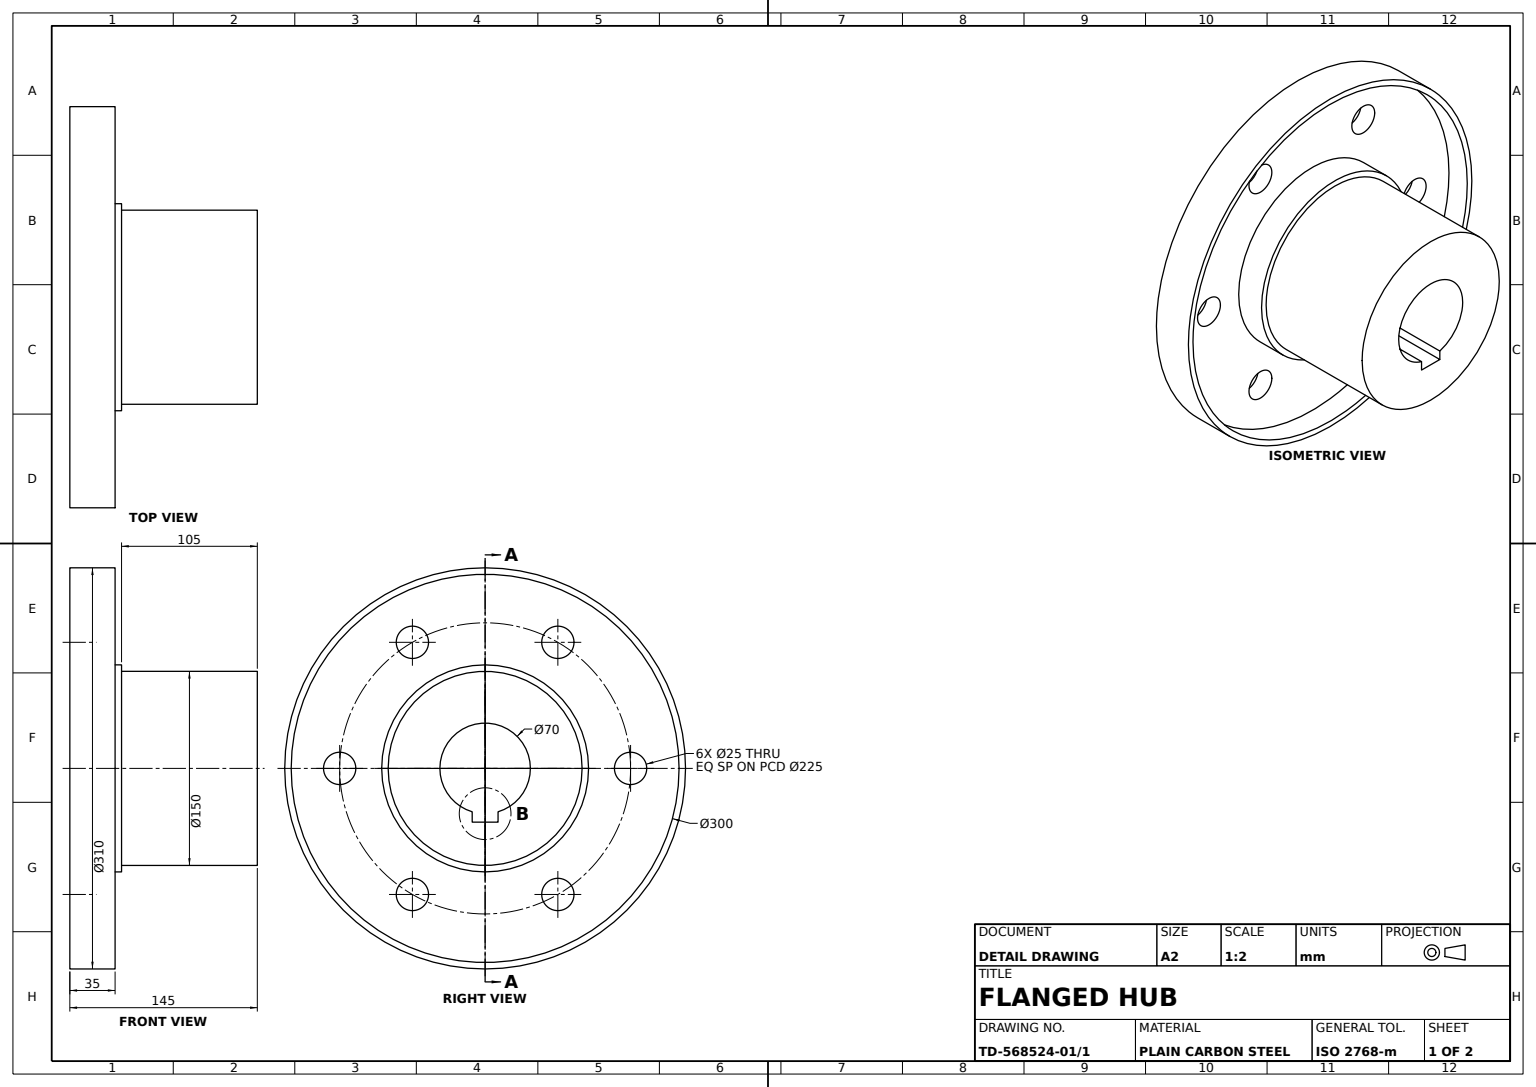
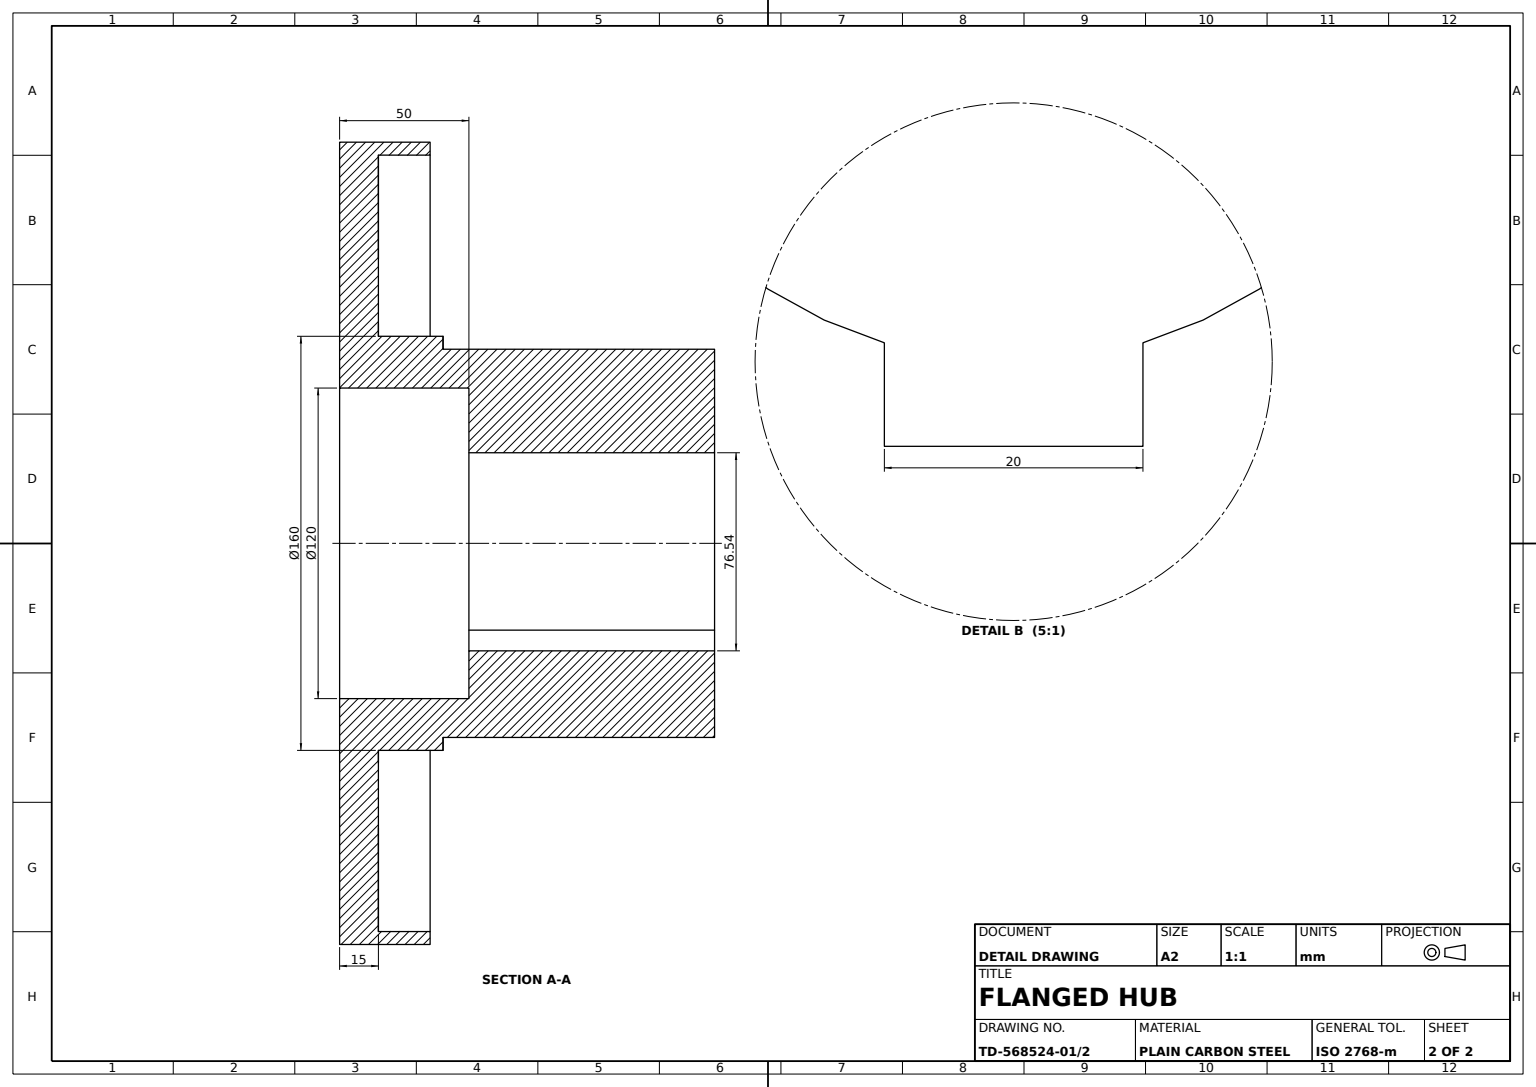
from build123d import *

# Parameters (mm, degrees)
FLANGE_RIM_SKETCH_R              = 155
FLANGE_RIM_SKETCH_R_2            = 150
FLANGE_RIM_310_DEPTH             = 35
FLANGE_BASE_SKETCH_R             = 150
FLANGE_BASE_DISC_DEPTH           = 15
MOUNTING_HOLES_SKETCH_R          = 12.5
MOUNTING_HOLES_6X_DEPTH          = 65
HUB_SHOULDER_SKETCH_R            = 80
HUB_SHOULDER_160_DEPTH           = 25
HUB_SKETCH_R                     = 75
HUB_150_DEPTH                    = 105
KEYED_BORE_WITH_KEYWAY_8X8_DEPTH = 142
RECESS_SKETCH_R                  = 60
RECESS_120_DEPTH                 = 50


with BuildPart() as part:
    # Flange Rim Sketch → Flange Rim Ø310 (new body)
    with BuildSketch(Plane(origin=(0, 0, 0), x_dir=(1, 0, 0), z_dir=(0, 1, 0))):
        with Locations(Location((0, 0, 0), (0, 0, 270))):
            Circle(FLANGE_RIM_SKETCH_R)
        with Locations(Location((0, 0, 0), (0, 0, 270))):
            Circle(FLANGE_RIM_SKETCH_R_2, mode=Mode.SUBTRACT)
    extrude(amount=FLANGE_RIM_310_DEPTH)

    # Flange Base Sketch → Flange Base Disc (add)
    with BuildSketch(Plane(origin=(0, 0, 0), x_dir=(1, 0, 0), z_dir=(0, 1, 0))):
        with Locations(Location((0, 0, 0), (0, 0, 270))):
            Circle(FLANGE_BASE_SKETCH_R)
    extrude(amount=FLANGE_BASE_DISC_DEPTH)

    # Mounting Holes Sketch → Mounting Holes 6x (cut)
    with BuildSketch(Plane(origin=(0, 15, 0), x_dir=(1, 0, 0), z_dir=(0, 1, 0))):
        with Locations(Location((0, 112.5, 0), (0, 0, 270))):
            Circle(MOUNTING_HOLES_SKETCH_R)
        with Locations(Location((97.427857926, 56.25, 0), (0, 0, 270))):
            Circle(MOUNTING_HOLES_SKETCH_R)
        with Locations(Location((97.427857926, -56.25, 0), (0, 0, 270))):
            Circle(MOUNTING_HOLES_SKETCH_R)
        with Locations(Location((0, -112.5, 0), (0, 0, 270))):
            Circle(MOUNTING_HOLES_SKETCH_R)
        with Locations(Location((-97.427857926, -56.25, 0), (0, 0, 270))):
            Circle(MOUNTING_HOLES_SKETCH_R)
        with Locations(Location((-97.427857926, 56.25, 0), (0, 0, 270))):
            Circle(MOUNTING_HOLES_SKETCH_R)
    extrude(amount=-MOUNTING_HOLES_6X_DEPTH, mode=Mode.SUBTRACT)

    # Hub Shoulder Sketch → Hub Shoulder Ø160 (add)
    with BuildSketch(Plane(origin=(0, 15, 0), x_dir=(1, 0, 0), z_dir=(0, 1, 0))):
        with Locations(Location((0, 0, 0), (0, 0, 270))):
            Circle(HUB_SHOULDER_SKETCH_R)
    extrude(amount=HUB_SHOULDER_160_DEPTH)

    # Hub Sketch → Hub Ø150 (add)
    with BuildSketch(Plane(origin=(0, 40, 0), x_dir=(1, 0, 0), z_dir=(0, 1, 0))):
        with Locations(Location((0, 0, 0), (0, 0, 270))):
            Circle(HUB_SKETCH_R)
    extrude(amount=HUB_150_DEPTH)

    # Keyed Bore Sketch → Keyed Bore with Keyway 8x8 (cut)
    with BuildSketch(Plane(origin=(0, 145, 0), x_dir=(1, 0, 0), z_dir=(0, 1, 0))):
        with BuildLine():
            Line((41.541019662, 10), (33.541019662, 10))
            ThreePointArc((33.541019662, 10), (-35, 0), (33.541019662, -10))
            Line((33.541019662, -10), (41.541019662, -10))
            Line((41.541019662, -10), (41.541019662, 10))
        make_face()
    extrude(amount=-KEYED_BORE_WITH_KEYWAY_8X8_DEPTH, mode=Mode.SUBTRACT)

    # Recess Sketch → Recess Ø120 (cut)
    with BuildSketch(Plane.XZ):
        with Locations(Location((0, 0, 0), (0, 0, 270))):
            Circle(RECESS_SKETCH_R)
    extrude(amount=-RECESS_120_DEPTH, mode=Mode.SUBTRACT)


solid = part.part
